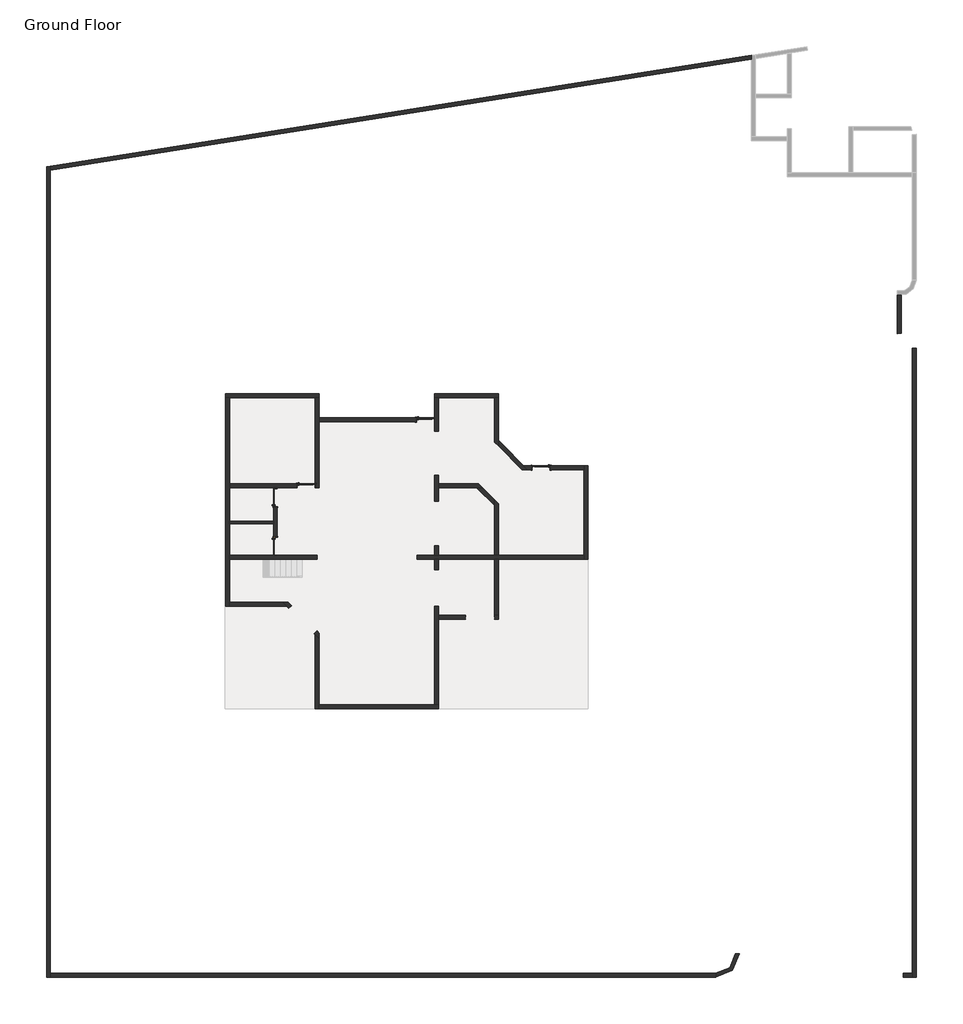
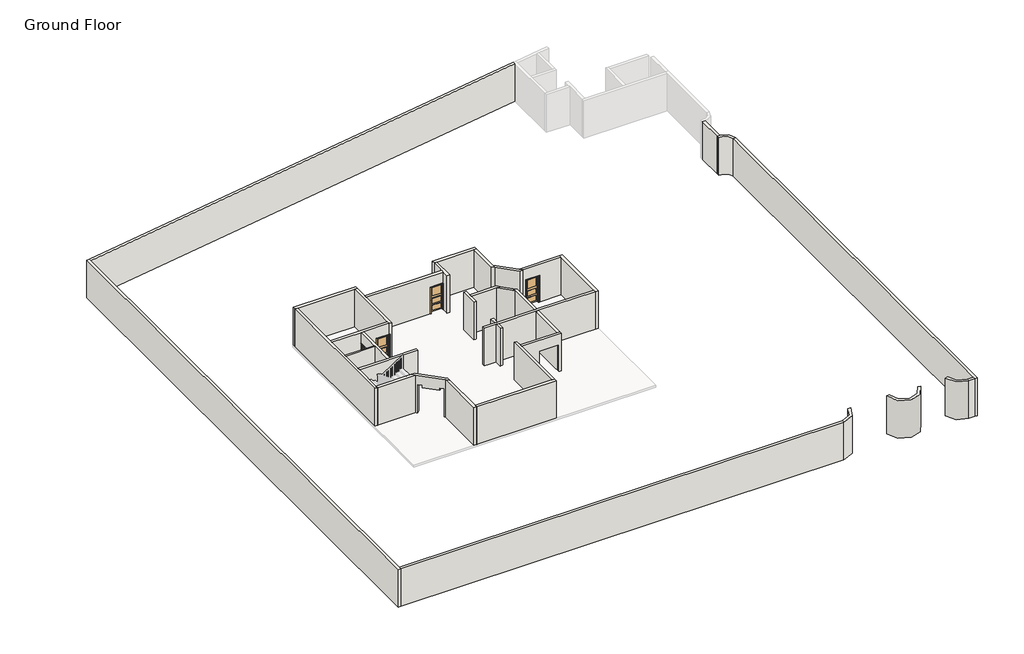
# One storey, part 1 of 2: 37 walls, 5 doors.
"""IFC4 building model written with IfcOpenShell, lengths in millimetres."""

from ifc_helpers import new_model, si_unit, point, frame, frame_2d, origin, origin_with_axes, place, context, project, spatial, polyline, circle_curve, trimmed, segment, composite_curve, outline, extrude, faceted_brep, transform, mapped, element, save
from ifc_brep_helpers import plane_surface, cylinder_surface, revolved_surface, advanced_brep
from components import door_9c4ddfbd, door_1a936fe1, door_721a2355, door_ac5ca1ae

model = new_model("IFC4")

# Units and contexts
model_context = context("Model", 3, world=origin())
ifc_project = project(units=[si_unit("LENGTHUNIT", "METRE", prefix="MILLI")], contexts=[model_context])

# Site, building, storey
site = spatial("IfcSite", under=ifc_project)
building = spatial("IfcBuilding", under=site)
storey = spatial("IfcBuildingStorey", under=building, Name="Ground Floor", Elevation=0.0)

# Doors
placement = place(None, origin())
door_shape = door_9c4ddfbd(model_context)
element("IfcDoor", 1, ObjectType="Door-Interior-Single-1_Panel-Wood : 36\" x 84\"", at=placement, inside=storey, context=model_context, shape_type="MappedRepresentation", body=[
    mapped(door_shape, transform((-23510.5118183, 2144.5392873, 0.0), x_axis=(0.0, 1.0, 0.0), y_axis=(-1.0, 0.0, 0.0), z_axis=(0.0, 0.0, 1.0))),
])
door_2_shape = door_1a936fe1(model_context)
element("IfcDoor", 2, ObjectType="Door-Interior-Single-1_Panel-Wood : 36\" x 84\"", at=placement, inside=storey, context=model_context, shape_type="MappedRepresentation", body=[
    mapped(door_2_shape, transform((-23510.5118183, -342.9715416, 0.0), x_axis=(0.0, -1.0, 0.0), y_axis=(1.0, 0.0, 0.0), z_axis=(0.0, 0.0, 1.0))),
])
door_3_shape = door_721a2355(model_context)
element("IfcDoor", 3, ObjectType="Door-Interior-Single-3_Panel_Vert-Wood : 3' x 6'11\" D1", at=placement, inside=storey, context=model_context, shape_type="MappedRepresentation", body=[
    mapped(door_3_shape, transform((-21930.4431154, 2757.3142873, 0.0), x_axis=(1.0, 0.0, 0.0), y_axis=(0.0, 1.0, 0.0), z_axis=(0.0, 0.0, 1.0))),
])
element("IfcDoor", 4, ObjectType="Door-Interior-Single-3_Panel_Vert-Wood : 3' x 6'11\" D1", at=placement, inside=storey, context=model_context, shape_type="MappedRepresentation", body=[
    mapped(door_3_shape, transform((-15845.1112935, 6113.4026825, 0.0), x_axis=(1.0, 0.0, 0.0), y_axis=(0.0, 1.0, 0.0), z_axis=(0.0, 0.0, 1.0))),
])
door_4_shape = door_ac5ca1ae(model_context)
element("IfcDoor", 5, ObjectType="Door-Interior-Single-3_Panel_Vert-Wood : 3' x 6'11\" D1", at=placement, inside=storey, context=model_context, shape_type="MappedRepresentation", body=[
    mapped(door_4_shape, transform((-9949.3197767, 3672.6109048, 0.0), x_axis=(-1.0, 0.0, 0.0), y_axis=(0.0, -1.0, 0.0), z_axis=(0.0, 0.0, 1.0))),
])

# Walls
element("IfcWall", 6, ObjectType="Generic - 0' - 4 15/16\"", at=placement, inside=storey, context=model_context, shape_type="SweptSolid", body=[
    extrude(outline(polyline([(-23608.9368183, 805.292672), (-25842.0443119, 805.292672), (-25842.0443119, 930.705172), (-23608.9368183, 930.705172), (-23608.9368183, 805.292672)])), origin_with_axes(), (0.0, 0.0, 1.0), 3048.0),
])
element("IfcWall", 7, ObjectType="Generic - 0' - 7 15/16\"", at=placement, inside=storey, context=model_context, shape_type="Brep", body=[
    faceted_brep([(9195.0010201, -22328.4007574, 0.0), (9195.0010201, 9753.6969485, 0.0), (9195.0010201, 9753.6969485, 3048.0), (9195.0010201, -22328.4007574, 3048.0), (8993.3885201, -22328.4007574, 0.0), (8993.3885201, -22328.4007574, 3048.0), (8993.3885201, -22126.7882574, 3048.0), (8993.3885201, 9747.3880188, 3048.0), (8993.3885201, 9747.3880188, 0.0), (8993.3885201, -22126.7882574, 0.0)], [[[0, 1, 2, 3]], [[4, 5, 6, 7, 8, 9]], [[1, 0, 4, 9, 8]], [[3, 2, 7, 6, 5]], [[2, 1, 8, 7]], [[0, 3, 5, 4]]]),
])
element("IfcWall", 8, ObjectType="Generic - 0' - 7 15/16\"", at=placement, inside=storey, context=model_context, shape_type="AdvancedBrep", body=[
    advanced_brep(
    [(9195.0010201, 9753.6969485, 3048.0), (8420.3375232, 10522.820987, 3048.0), (8218.7317611, 10508.1549201, 3048.0), (8218.7317611, 10301.2352695, 3048.0), (8993.3885201, 9747.3880188, 3048.0), (9195.0010201, 9753.6969485, 0.0), (8993.3885201, 9747.3880188, 0.0), (8218.7317611, 10301.2352695, 0.0), (8218.7317611, 10508.1549201, 0.0), (8420.3375232, 10522.820987, 0.0)],
    [
        (0, 1, circle_curve(frame((8378.4275035, 9705.9257341, 3048.0), z_axis=(0.0, 0.0, 1.0), x_axis=(1.0, 0.0, 0.0)), 817.9696798)),
        (1, 2, circle_curve(frame((8378.4275035, 9705.9257341, 3048.0), z_axis=(0.0, 0.0, 1.0), x_axis=(1.0, 0.0, 0.0)), 817.9696229)),
        (2, 3),
        (3, 4, circle_curve(frame((8378.4275035, 9705.9257341, 3048.0), z_axis=(0.0, 0.0, -1.0), x_axis=(1.0, 0.0, 0.0)), 616.3571798)),
        (4, 0),
        (5, 6),
        (6, 7, circle_curve(frame((8378.4275035, 9705.9257341, 0.0), z_axis=(0.0, 0.0, 1.0), x_axis=(1.0, 0.0, 0.0)), 616.3571798)),
        (7, 8),
        (8, 9, circle_curve(frame((8378.4275035, 9705.9257341, 0.0), z_axis=(0.0, 0.0, -1.0), x_axis=(1.0, 0.0, 0.0)), 817.9696798)),
        (9, 5, circle_curve(frame((8378.4275035, 9705.9257341, 0.0), z_axis=(0.0, 0.0, -1.0), x_axis=(1.0, 0.0, 0.0)), 817.9696229)),
        (0, 5),
        (8, 2),
        (3, 7),
        (6, 4),
    ],
    [
        plane_surface(frame((9196.3971832, 9705.9257341, 3048.0), z_axis=(0.0, 0.0, 1.0), x_axis=(0.0, 1.0, 0.0))),
        plane_surface(frame((9196.3971832, 9705.9257341, 0.0), z_axis=(0.0, 0.0, -1.0), x_axis=(0.0, -1.0, 0.0))),
        cylinder_surface(frame((8378.4275035, 9705.9257341, 0.0), z_axis=(0.0, 0.0, 1.0), x_axis=(1.0, 0.0, 0.0)), 817.9696798),
        revolved_surface(polyline([(8994.784683299999, 9705.9257341, 0.0), (8994.784683299999, 9705.9257341, 3048.0)]), (8378.4275035, 9705.9257341, 0.0), (0.0, 0.0, -1.0)),
        plane_surface(frame((8993.3885201, 9747.3880188, 0.0), z_axis=(0.03127704426469031, -0.9995107535699977, 0.0), x_axis=(0.9995107535699977, 0.03127704426469031, 0.0))),
        plane_surface(frame((8218.7317611, 12658.7719349, 0.0), z_axis=(-1.0, 0.0, 0.0), x_axis=(0.0, -1.0, 0.0))),
    ],
    [
        (0, [[1, 2, 3, 4, 5]]),
        (1, [[6, 7, 8, 9, 10]]),
        (2, [[-2, -1, 11, -10, -9, 12]]),
        (3, [[-4, 13, -7, 14]]),
        (4, [[-5, -14, -6, -11]]),
        (5, [[-3, -12, -8, -13]]),
    ],
),
])
element("IfcWall", 9, ObjectType="Generic - 0' - 7 15/16\"", at=placement, inside=storey, context=model_context, shape_type="SweptSolid", body=[
    extrude(outline(composite_curve([segment(polyline([(8218.7317611, 10508.1549201), (8218.7317611, 12472.8269263)]), True, "CONTINUOUS"), segment(trimmed(circle_curve(frame_2d((8381.1692405, 13271.1676702)), 814.6986425), [point((8218.7317611, 12472.8269263))], [point((8420.3442611, 12457.4114439))], True, "CARTESIAN"), True, "CONTINUOUS"), segment(polyline([(8420.3442611, 12457.4114439), (8420.3442611, 10522.8206982)]), True, "CONTINUOUS"), segment(trimmed(circle_curve(frame_2d((8378.4275035, 9705.9257341)), 817.9696798), [point((8420.3442611, 10522.8206982))], [point((8218.7317611, 10508.1549201))], True, "CARTESIAN"), True, "CONTINUOUS")], self_intersect=False)), origin_with_axes(), (0.0, 0.0, 1.0), 3048.0),
])
element("IfcWall", 10, ObjectType="Generic - 0' - 7 15/16\"", at=placement, inside=storey, context=model_context, shape_type="SweptSolid", body=[
    extrude(outline(polyline([(8993.3885201, -22328.4007574), (8533.7347238, -22328.4007574), (8535.4479834, -22126.7882574), (8993.3885201, -22126.7882574), (8993.3885201, -22328.4007574)])), origin_with_axes(), (0.0, 0.0, 1.0), 3048.0),
])
element("IfcWall", 11, ObjectType="Generic - 0' - 7 15/16\"", at=placement, inside=storey, context=model_context, shape_type="SweptSolid", body=[
    extrude(outline(composite_curve([segment(polyline([(7335.4391325, -21276.4548413), (7534.9019602, -21247.0919307)]), True, "CONTINUOUS"), segment(trimmed(circle_curve(frame_2d((8553.7677892, -21097.104755)), 1029.8464596), [point((7534.9019602, -21247.0919307))], [point((8535.4479834, -22126.7882574))], True, "CARTESIAN"), True, "CONTINUOUS"), segment(polyline([(8535.4479834, -22126.7882574), (8533.7347238, -22328.4007574)]), True, "CONTINUOUS"), segment(trimmed(circle_curve(frame_2d((8553.7677892, -21097.104755)), 1231.4589596), [point((8533.7347238, -22328.4007574))], [point((7335.4391325, -21276.4548413))], False, "CARTESIAN"), True, "CONTINUOUS")], self_intersect=False)), origin_with_axes(), (0.0, 0.0, 1.0), 3048.0),
])
element("IfcWall", 12, ObjectType="Generic - 0' - 7 15/16\"", at=placement, inside=storey, context=model_context, shape_type="SweptSolid", body=[
    extrude(outline(composite_curve([segment(polyline([(2932.0157835, -21122.0907213), (3133.3995752, -21112.4902743)]), True, "CONTINUOUS"), segment(trimmed(circle_curve(frame_2d((4193.0797295, -21061.9727873)), 1060.8836156), [point((3133.3995752, -21112.4902743))], [point((5237.6872867, -21247.0919307))], True, "CARTESIAN"), True, "CONTINUOUS"), segment(polyline([(5237.6872867, -21247.0919307), (5436.2066512, -21282.2723527)]), True, "CONTINUOUS"), segment(trimmed(circle_curve(frame_2d((4193.0797295, -21061.9727873)), 1262.4961156), [point((5436.2066512, -21282.2723527))], [point((2932.0157835, -21122.0907213))], False, "CARTESIAN"), True, "CONTINUOUS")], self_intersect=False)), origin_with_axes(), (0.0, 0.0, 1.0), 3048.0),
])
element("IfcWall", 13, ObjectType="Generic - 0' - 7 15/16\"", at=placement, inside=storey, context=model_context, shape_type="SweptSolid", body=[
    extrude(outline(composite_curve([segment(polyline([(-1043.7652203, -22328.1084547), (-1043.7652203, -22126.4959547)]), True, "CONTINUOUS"), segment(trimmed(circle_curve(frame_2d((-1043.7652203, -21112.4902743)), 1014.0056804), [point((-1043.7652203, -22126.4959547))], [point((-29.7595399, -21112.4902743))], True, "CARTESIAN"), True, "CONTINUOUS"), segment(polyline([(-29.7595399, -21112.4902743), (171.8529601, -21112.4902743)]), True, "CONTINUOUS"), segment(trimmed(circle_curve(frame_2d((-1043.7652203, -21112.4902743)), 1215.6181804), [point((171.8529601, -21112.4902743))], [point((-1043.7652203, -22328.1084547))], False, "CARTESIAN"), True, "CONTINUOUS")], self_intersect=False)), origin_with_axes(), (0.0, 0.0, 1.0), 3048.0),
])
element("IfcWall", 14, ObjectType="Generic - 0' - 7 15/16\"", at=placement, inside=storey, context=model_context, shape_type="Brep", body=[
    faceted_brep([(-35183.4613906, 19002.9774571, 0.0), (-35183.4613906, -22328.4007574, 0.0), (-35183.4613906, -22328.4007574, 3048.0), (-35183.4613906, 19002.9774571, 3048.0), (-34981.8488906, 19034.9188254, 0.0), (-34981.8488906, 19034.9188254, 3048.0), (-34981.8488906, 18830.7917788, 3048.0), (-34981.8488906, -22328.4007574, 3048.0), (-34981.8488906, -22328.4007574, 0.0), (-34981.8488906, 18830.7917788, 0.0)], [[[0, 1, 2, 3]], [[4, 5, 6, 7, 8, 9]], [[1, 0, 4, 9, 8]], [[2, 1, 8, 7]], [[3, 2, 7, 6, 5]], [[0, 3, 5, 4]]]),
])
element("IfcWall", 15, ObjectType="Generic - 0' - 7 15/16\"", at=placement, inside=storey, context=model_context, shape_type="SweptSolid", body=[
    extrude(outline(polyline([(-1034.7920906, -22328.4007574), (-34981.5566627, -22328.4007574), (-34981.5566627, -22126.7882574), (-1034.7920906, -22126.7882574), (-1034.7920906, -22328.4007574)])), origin_with_axes(), (0.0, 0.0, 1.0), 3048.0),
])
element("IfcWall", 16, ObjectType="Generic - 0' - 7 15/16\"", at=placement, inside=storey, context=model_context, shape_type="Brep", body=[
    faceted_brep([(787.1202427, 24701.7788574, 0.0), (-34981.8488906, 19034.9188254, 0.0), (-34981.8488906, 19034.9188254, 3048.0), (787.1202427, 24701.7788574, 3048.0), (787.1202427, 24497.6518108, 0.0), (787.1202427, 24497.6518108, 3048.0), (-34981.8488906, 18830.7917788, 3048.0), (-34981.8488906, 18830.7917788, 0.0), (787.1202427, 24699.1003289, 0.0), (787.1202427, 24699.1003289, 3048.0)], [[[0, 1, 2, 3]], [[4, 5, 6, 7]], [[1, 0, 8, 4, 7]], [[3, 2, 6, 5, 9]], [[0, 3, 9, 5, 4, 8]], [[2, 1, 7, 6]]]),
])
element("IfcWall", 17, ObjectType="Generic - 0' - 7 15/16\"", at=placement, inside=storey, context=model_context, shape_type="Brep", body=[
    faceted_brep([(-25842.0443119, -800.9652916, 3048.0), (-23608.9368183, -800.9652916, 3048.0), (-23405.7368183, -800.9652916, 3048.0), (-21373.2387805, -800.9652916, 3048.0), (-21373.2387805, -800.9652916, 0.0), (-23405.7368183, -800.9652916, 0.0), (-23405.7368183, -800.9652916, 2159.0), (-23608.9368183, -800.9652916, 2159.0), (-23608.9368183, -800.9652916, 0.0), (-25842.0443119, -800.9652916, 0.0), (-25842.0443119, -1002.5777916, 0.0), (-21373.2387805, -1002.5777916, 0.0), (-21373.2387805, -1002.5777916, 3048.0), (-25842.0443119, -1002.5777916, 3048.0), (-23608.9368183, -825.5715416, 0.0), (-23405.7368183, -825.5715416, 0.0), (-23608.9368183, -825.5715416, 2159.0), (-23405.7368183, -825.5715416, 2159.0)], [[[0, 1, 2, 3, 4, 5, 6, 7, 8, 9]], [[10, 11, 12, 13]], [[11, 10, 9, 8, 14, 15, 5, 4]], [[3, 2, 1, 0, 13, 12]], [[4, 3, 12, 11]], [[0, 9, 10, 13]], [[16, 14, 8, 7]], [[15, 17, 6, 5]], [[14, 16, 17, 15]], [[17, 16, 7, 6]]]),
])
element("IfcWall", 18, ObjectType="Generic - 8\"", at=placement, inside=storey, context=model_context, shape_type="Brep", body=[
    faceted_brep([(-21270.0431154, 7427.7381656, 0.0), (-26045.2443119, 7427.7381656, 0.0), (-26045.2443119, 7427.7381656, 3048.0), (-21270.0431154, 7427.7381656, 3048.0), (-21270.0431154, 7224.5381656, 0.0), (-21270.0431154, 7224.5381656, 3048.0), (-21473.2431154, 7224.5381656, 3048.0), (-25842.0443119, 7224.5381656, 3048.0), (-26045.2443119, 7224.5381656, 3048.0), (-26045.2443119, 7224.5381656, 0.0), (-25842.0443119, 7224.5381656, 0.0), (-21473.2431154, 7224.5381656, 0.0)], [[[0, 1, 2, 3]], [[4, 5, 6, 7, 8, 9, 10, 11]], [[1, 0, 4, 11, 10, 9]], [[3, 2, 8, 7, 6, 5]], [[2, 1, 9, 8]], [[0, 3, 5, 4]]]),
])
element("IfcWall", 19, ObjectType="Generic - 8\"", at=placement, inside=storey, context=model_context, shape_type="Brep", body=[
    faceted_brep([(-25842.0443119, -3391.115973, 0.0), (-25842.0443119, -3187.915973, 0.0), (-25842.0443119, -1002.5777916, 0.0), (-25842.0443119, -800.9652916, 0.0), (-25842.0443119, 805.292672, 0.0), (-25842.0443119, 930.705172, 0.0), (-25842.0443119, 2652.5392873, 0.0), (-25842.0443119, 2855.7392873, 0.0), (-25842.0443119, 7224.5381656, 0.0), (-25842.0443119, 7224.5381656, 3048.0), (-25842.0443119, 2855.7392873, 3048.0), (-25842.0443119, 2652.5392873, 3048.0), (-25842.0443119, 930.705172, 3048.0), (-25842.0443119, 805.292672, 3048.0), (-25842.0443119, -800.9652916, 3048.0), (-25842.0443119, -1002.5777916, 3048.0), (-25842.0443119, -3187.915973, 3048.0), (-25842.0443119, -3391.115973, 3048.0), (-26045.2443119, -3391.115973, 0.0), (-26045.2443119, -3391.115973, 3048.0), (-26045.2443119, 7224.5381656, 3048.0), (-26045.2443119, 7224.5381656, 0.0)], [[[0, 1, 2, 3, 4, 5, 6, 7, 8, 9, 10, 11, 12, 13, 14, 15, 16, 17]], [[18, 19, 20, 21]], [[8, 7, 6, 5, 4, 3, 2, 1, 0, 18, 21]], [[17, 16, 15, 14, 13, 12, 11, 10, 9, 20, 19]], [[9, 8, 21, 20]], [[0, 17, 19, 18]]]),
])
element("IfcWall", 20, ObjectType="Generic - 8\"", at=placement, inside=storey, context=model_context, shape_type="Brep", body=[
    faceted_brep([(-25842.0443119, 2855.7392873, 3048.0), (-21473.2431154, 2855.7392873, 3048.0), (-21473.2431154, 2855.7392873, 2133.6), (-22413.0431154, 2855.7392873, 2133.6), (-22413.0431154, 2855.7392873, 0.0), (-25842.0443119, 2855.7392873, 0.0), (-21473.2431154, 2652.5392873, 3048.0), (-23405.7368183, 2652.5392873, 3048.0), (-23608.9368183, 2652.5392873, 3048.0), (-25842.0443119, 2652.5392873, 3048.0), (-25842.0443119, 2652.5392873, 0.0), (-23608.9368183, 2652.5392873, 0.0), (-23405.7368183, 2652.5392873, 0.0), (-22413.0431154, 2652.5392873, 0.0), (-22413.0431154, 2652.5392873, 2133.6), (-21473.2431154, 2652.5392873, 2133.6)], [[[0, 1, 2, 3, 4, 5]], [[6, 7, 8, 9, 10, 11, 12, 13, 14, 15]], [[10, 5, 4, 13, 12, 11]], [[1, 0, 9, 8, 7, 6]], [[0, 5, 10, 9]], [[1, 6, 15, 2]], [[14, 3, 2, 15]], [[3, 14, 13, 4]]]),
])
element("IfcWall", 21, ObjectType="Generic - 8\"", at=placement, inside=storey, context=model_context, shape_type="Brep", body=[
    faceted_brep([(-21270.0431154, 2652.5392873, 0.0), (-21270.0431154, 6008.6276825, 0.0), (-21270.0431154, 6211.8276825, 0.0), (-21270.0431154, 7224.5381656, 0.0), (-21270.0431154, 7224.5381656, 3048.0), (-21270.0431154, 6211.8276825, 3048.0), (-21270.0431154, 6008.6276825, 3048.0), (-21270.0431154, 2652.5392873, 3048.0), (-21473.2431154, 2652.5392873, 3048.0), (-21473.2431154, 2855.7392873, 3048.0), (-21473.2431154, 7224.5381656, 3048.0), (-21473.2431154, 7224.5381656, 0.0), (-21473.2431154, 2855.7392873, 0.0), (-21473.2431154, 2855.7392873, 2133.6), (-21473.2431154, 2652.5392873, 2133.6), (-21447.8431154, 2652.5392873, 0.0), (-21447.8431154, 2855.7392873, 0.0), (-21447.8431154, 2652.5392873, 2133.6), (-21447.8431154, 2855.7392873, 2133.6)], [[[0, 1, 2, 3, 4, 5, 6, 7]], [[8, 9, 10, 11, 12, 13, 14]], [[3, 2, 1, 0, 15, 16, 12, 11]], [[7, 6, 5, 4, 10, 9, 8]], [[4, 3, 11, 10]], [[0, 7, 8, 14, 17, 15]], [[16, 18, 13, 12]], [[18, 16, 15, 17]], [[18, 17, 14, 13]]]),
])
element("IfcWall", 22, ObjectType="Generic - 8\"", at=placement, inside=storey, context=model_context, shape_type="SweptSolid", body=[
    extrude(outline(polyline([(3048.0, -15387.9112935), (3048.0, -21270.0431154), (0.0, -21270.0431154), (0.0, -16327.7112935), (2133.6, -16327.7112935), (2133.6, -15387.9112935), (3048.0, -15387.9112935)])), frame((0.0, 6008.6276825, 0.0), z_axis=(0.0, 1.0, 0.0), x_axis=(0.0, 0.0, 1.0)), (0.0, 0.0, 1.0), 203.2),
])
element("IfcWall", 23, ObjectType="Generic - 8\"", at=placement, inside=storey, context=model_context, shape_type="SweptSolid", body=[
    extrude(outline(polyline([(-15177.0356792, 7224.5381656), (-15177.0356792, 5525.355182), (-15380.2356792, 5525.355182), (-15380.2356792, 7224.5381656), (-15177.0356792, 7224.5381656)])), origin_with_axes(), (0.0, 0.0, 1.0), 3048.0),
])
element("IfcWall", 24, ObjectType="Generic - 8\"", at=placement, inside=storey, context=model_context, shape_type="Brep", body=[
    faceted_brep([(-12130.529643, 7427.7381656, 0.0), (-15383.4246912, 7427.7381656, 0.0), (-15383.4246912, 7427.7381656, 3048.0), (-12130.529643, 7427.7381656, 3048.0), (-12130.529643, 7224.5381656, 0.0), (-12130.529643, 7224.5381656, 3048.0), (-12133.7209731, 7224.5381656, 3048.0), (-12336.9209731, 7224.5381656, 3048.0), (-15177.0356792, 7224.5381656, 3048.0), (-15380.2356792, 7224.5381656, 3048.0), (-15383.4246912, 7224.5381656, 3048.0), (-15383.4246912, 7224.5381656, 0.0), (-15380.2356792, 7224.5381656, 0.0), (-15177.0356792, 7224.5381656, 0.0), (-12336.9209731, 7224.5381656, 0.0), (-12133.7209731, 7224.5381656, 0.0)], [[[0, 1, 2, 3]], [[4, 5, 6, 7, 8, 9, 10, 11, 12, 13, 14, 15]], [[1, 0, 4, 15, 14, 13, 12, 11]], [[2, 1, 11, 10]], [[3, 2, 10, 9, 8, 7, 6, 5]], [[0, 3, 5, 4]]]),
])
element("IfcWall", 25, ObjectType="Generic - 8\"", at=placement, inside=storey, context=model_context, shape_type="Brep", body=[
    faceted_brep([(-12133.7209731, 4774.4410298, 0.0), (-10927.1158481, 3567.8359048, 0.0), (-10927.1158481, 3567.8359048, 3048.0), (-12133.7209731, 4774.4410298, 3048.0), (-12133.7209731, 5061.8092257, 0.0), (-12133.7209731, 5061.8092257, 3048.0), (-10842.9476523, 3771.0359048, 3048.0), (-10639.7476523, 3567.8359048, 3048.0), (-10639.7476523, 3567.8359048, 0.0), (-10842.9476523, 3771.0359048, 0.0)], [[[0, 1, 2, 3]], [[4, 5, 6, 7, 8, 9]], [[1, 0, 4, 9, 8]], [[3, 2, 7, 6, 5]], [[2, 1, 8, 7]], [[0, 3, 5, 4]]]),
])
element("IfcWall", 26, ObjectType="Generic - 8\"", at=placement, inside=storey, context=model_context, shape_type="Brep", body=[
    faceted_brep([(-12336.9209731, 7224.5381656, 0.0), (-12336.9209731, 4977.6410298, 0.0), (-12336.9209731, 4977.6410298, 3048.0), (-12336.9209731, 7224.5381656, 3048.0), (-12133.7209731, 7224.5381656, 0.0), (-12133.7209731, 7224.5381656, 3048.0), (-12133.7209731, 5061.8092257, 3048.0), (-12133.7209731, 4774.4410298, 3048.0), (-12133.7209731, 4774.4410298, 0.0), (-12133.7209731, 5061.8092257, 0.0)], [[[0, 1, 2, 3]], [[4, 5, 6, 7, 8, 9]], [[1, 0, 4, 9, 8]], [[3, 2, 7, 6, 5]], [[2, 1, 8, 7]], [[0, 3, 5, 4]]]),
])
element("IfcWall", 27, ObjectType="Generic - 8\"", at=placement, inside=storey, context=model_context, shape_type="Brep", body=[
    faceted_brep([(-7764.9197767, 3771.0359048, 0.0), (-7764.9197767, 3567.8359048, 0.0), (-7764.9197767, -800.9652916, 0.0), (-7764.9197767, -1004.1652916, 0.0), (-7764.9197767, -1004.1652916, 3048.0), (-7764.9197767, -800.9652916, 3048.0), (-7764.9197767, 3567.8359048, 3048.0), (-7764.9197767, 3771.0359048, 3048.0), (-7561.7197767, 3771.0359048, 0.0), (-7561.7197767, 3771.0359048, 3048.0), (-7561.7197767, -1004.1652916, 3048.0), (-7561.7197767, -1004.1652916, 0.0)], [[[0, 1, 2, 3, 4, 5, 6, 7]], [[8, 9, 10, 11]], [[3, 2, 1, 0, 8, 11]], [[7, 6, 5, 4, 10, 9]], [[4, 3, 11, 10]], [[0, 7, 9, 8]]]),
])
element("IfcWall", 28, ObjectType="Generic - 8\"", at=placement, inside=storey, context=model_context, shape_type="Brep", body=[
    faceted_brep([(-7764.9197767, -800.9652916, 0.0), (-12130.529643, -800.9652916, 0.0), (-12333.729643, -800.9652916, 0.0), (-15177.0356792, -800.9652916, 0.0), (-15380.2356792, -800.9652916, 0.0), (-16280.7750494, -800.9652916, 0.0), (-16280.7750494, -800.9652916, 3048.0), (-15380.2356792, -800.9652916, 3048.0), (-15177.0356792, -800.9652916, 3048.0), (-12333.729643, -800.9652916, 3048.0), (-12130.529643, -800.9652916, 3048.0), (-7764.9197767, -800.9652916, 3048.0), (-7764.9197767, -1004.1652916, 0.0), (-7764.9197767, -1004.1652916, 3048.0), (-12130.529643, -1004.1652916, 3048.0), (-12333.729643, -1004.1652916, 3048.0), (-15177.0356792, -1004.1652916, 3048.0), (-15380.2356792, -1004.1652916, 3048.0), (-16280.7750494, -1004.1652916, 3048.0), (-16280.7750494, -1004.1652916, 0.0), (-15380.2356792, -1004.1652916, 0.0), (-15177.0356792, -1004.1652916, 0.0), (-12333.729643, -1004.1652916, 0.0), (-12130.529643, -1004.1652916, 0.0)], [[[0, 1, 2, 3, 4, 5, 6, 7, 8, 9, 10, 11]], [[12, 13, 14, 15, 16, 17, 18, 19, 20, 21, 22, 23]], [[5, 4, 3, 2, 1, 0, 12, 23, 22, 21, 20, 19]], [[6, 5, 19, 18]], [[11, 10, 9, 8, 7, 6, 18, 17, 16, 15, 14, 13]], [[0, 11, 13, 12]]]),
])
element("IfcWall", 29, ObjectType="Generic - 8\"", at=placement, inside=storey, context=model_context, shape_type="Brep", body=[
    faceted_brep([(-12130.529643, -800.9652916, 0.0), (-12130.529643, 1838.499171, 0.0), (-12130.529643, 1838.499171, 3048.0), (-12130.529643, -800.9652916, 3048.0), (-12333.729643, -800.9652916, 0.0), (-12333.729643, -800.9652916, 3048.0), (-12333.729643, 1754.3309751, 3048.0), (-12333.729643, 2041.699171, 3048.0), (-12333.729643, 2041.699171, 0.0), (-12333.729643, 1754.3309751, 0.0)], [[[0, 1, 2, 3]], [[4, 5, 6, 7, 8, 9]], [[1, 0, 4, 9, 8]], [[3, 2, 7, 6, 5]], [[0, 3, 5, 4]], [[2, 1, 8, 7]]]),
])
element("IfcWall", 30, ObjectType="Generic - 8\"", at=placement, inside=storey, context=model_context, shape_type="SweptSolid", body=[
    extrude(outline(polyline([(-12130.529643, -1004.1652916), (-12130.529643, -3846.1737377), (-12333.729643, -3846.1737377), (-12333.729643, -1004.1652916), (-12130.529643, -1004.1652916)])), origin_with_axes(), (0.0, 0.0, 1.0), 3048.0),
])
element("IfcWall", 31, ObjectType="Generic - 8\"", at=placement, inside=storey, context=model_context, shape_type="Brep", body=[
    faceted_brep([(-12130.529643, -4049.3737377, 3048.0), (-15180.2246912, -4049.3737377, 3048.0), (-15180.2246912, -4049.3737377, 0.0), (-13812.829643, -4049.3737377, 0.0), (-13812.829643, -4049.3737377, 2189.5), (-12327.829643, -4049.3737377, 2189.5), (-12327.829643, -4049.3737377, 0.0), (-12130.529643, -4049.3737377, 0.0), (-15180.2246912, -3846.1737377, 3048.0), (-12333.729643, -3846.1737377, 3048.0), (-12130.529643, -3846.1737377, 3048.0), (-12130.529643, -3846.1737377, 0.0), (-12327.829643, -3846.1737377, 0.0), (-12327.829643, -3846.1737377, 2189.5), (-13812.829643, -3846.1737377, 2189.5), (-13812.829643, -3846.1737377, 0.0), (-15180.2246912, -3846.1737377, 0.0), (-13812.829643, -3952.3737377, 0.0), (-13827.829643, -3952.3737377, 0.0), (-13827.829643, -4029.3737377, 0.0), (-13812.829643, -4029.3737377, 0.0), (-12327.829643, -4029.3737377, 0.0), (-12312.829643, -4029.3737377, 0.0), (-12312.829643, -3952.3737377, 0.0), (-12327.829643, -3952.3737377, 0.0), (-13812.829643, -4029.3737377, 2189.5), (-12327.829643, -4029.3737377, 2189.5), (-13827.829643, -4029.3737377, 2204.5), (-12312.829643, -4029.3737377, 2204.5), (-13827.829643, -3952.3737377, 2204.5), (-13812.829643, -3952.3737377, 2189.5), (-12327.829643, -3952.3737377, 2189.5), (-12312.829643, -3952.3737377, 2204.5)], [[[0, 1, 2, 3, 4, 5, 6, 7]], [[8, 9, 10, 11, 12, 13, 14, 15, 16]], [[2, 16, 15, 17, 18, 19, 20, 3]], [[11, 7, 6, 21, 22, 23, 24, 12]], [[1, 0, 10, 9, 8]], [[2, 1, 8, 16]], [[0, 7, 11, 10]], [[20, 25, 4, 3]], [[26, 21, 6, 5]], [[25, 26, 5, 4]], [[25, 20, 19, 27, 28, 22, 21, 26]], [[27, 19, 18, 29]], [[29, 18, 17, 30, 31, 24, 23, 32]], [[28, 27, 29, 32]], [[22, 28, 32, 23]], [[30, 17, 15, 14]], [[24, 31, 13, 12]], [[31, 30, 14, 13]]]),
])
element("IfcWall", 32, ObjectType="Generic - 8\"", at=placement, inside=storey, context=model_context, shape_type="Brep", body=[
    faceted_brep([(-15383.4246912, -3394.3072284, 0.0), (-15383.4246912, -8414.9836039, 0.0), (-15383.4246912, -8414.9836039, 3048.0), (-15383.4246912, -3394.3072284, 3048.0), (-15180.2246912, -3394.3072284, 0.0), (-15180.2246912, -3394.3072284, 3048.0), (-15180.2246912, -3846.1737377, 3048.0), (-15180.2246912, -4049.3737377, 3048.0), (-15180.2246912, -8414.9836039, 3048.0), (-15180.2246912, -8414.9836039, 0.0), (-15180.2246912, -4049.3737377, 0.0), (-15180.2246912, -3846.1737377, 0.0)], [[[0, 1, 2, 3]], [[4, 5, 6, 7, 8, 9, 10, 11]], [[1, 0, 4, 11, 10, 9]], [[3, 2, 8, 7, 6, 5]], [[0, 3, 5, 4]], [[2, 1, 9, 8]]]),
])
element("IfcWall", 33, ObjectType="Generic - 8\"", at=placement, inside=storey, context=model_context, shape_type="Brep", body=[
    faceted_brep([(-15180.2246912, -8414.9836039, 0.0), (-15383.4246912, -8414.9836039, 0.0), (-21270.0431154, -8414.9836039, 0.0), (-21270.0431154, -8414.9836039, 3048.0), (-15383.4246912, -8414.9836039, 3048.0), (-15180.2246912, -8414.9836039, 3048.0), (-15180.2246912, -8618.1836039, 0.0), (-15180.2246912, -8618.1836039, 3048.0), (-21270.0431154, -8618.1836039, 3048.0), (-21270.0431154, -8618.1836039, 0.0)], [[[0, 1, 2, 3, 4, 5]], [[6, 7, 8, 9]], [[2, 1, 0, 6, 9]], [[5, 4, 3, 8, 7]], [[3, 2, 9, 8]], [[0, 5, 7, 6]]]),
])
element("IfcWall", 34, ObjectType="Generic - 8\"", at=placement, inside=storey, context=model_context, shape_type="Brep", body=[
    faceted_brep([(-21270.0431154, -8618.1836039, 0.0), (-21270.0431154, -8414.9836039, 0.0), (-21270.0431154, -5059.1070276, 0.0), (-21270.0431154, -5059.1070276, 3048.0), (-21270.0431154, -8414.9836039, 3048.0), (-21270.0431154, -8618.1836039, 3048.0), (-21473.2431154, -8618.1836039, 0.0), (-21473.2431154, -8618.1836039, 3048.0), (-21473.2431154, -4855.9070276, 3048.0), (-21473.2431154, -4855.9070276, 0.0)], [[[0, 1, 2, 3, 4, 5]], [[6, 7, 8, 9]], [[2, 1, 0, 6, 9]], [[5, 4, 3, 8, 7]], [[3, 2, 9, 8]], [[0, 5, 7, 6]]]),
])
element("IfcWall", 35, ObjectType="Generic - 8\"", at=placement, inside=storey, context=model_context, shape_type="SweptSolid", body=[
    extrude(outline(polyline([(-25842.0443119, -3187.915973), (-23141.23417, -3187.915973), (-22938.03417, -3391.115973), (-25842.0443119, -3391.115973), (-25842.0443119, -3187.915973)])), origin_with_axes(), (0.0, 0.0, 1.0), 3048.0),
])
element("IfcWall", 36, ObjectType="Generic - 8\"", at=placement, inside=storey, context=model_context, shape_type="Brep", body=[
    faceted_brep([(-22853.8659741, -3187.915973, 3048.0), (-21270.0431154, -4771.7388317, 3048.0), (-21270.0431154, -4771.7388317, 0.0), (-21385.3381768, -4656.4437704, 0.0), (-21385.3381768, -4656.4437704, 2286.0), (-21600.8643237, -4440.9176235, 2286.0), (-21600.8643237, -4440.9176235, 2108.2), (-22462.9689113, -3578.8130358, 2108.2), (-22462.9689113, -3578.8130358, 2286.0), (-22678.4950582, -3363.2868889, 2286.0), (-22678.4950582, -3363.2868889, 0.0), (-22853.8659741, -3187.915973, 0.0), (-21270.0431154, -5059.1070276, 3048.0), (-21473.2431154, -4855.9070276, 3048.0), (-22938.03417, -3391.115973, 3048.0), (-23141.23417, -3187.915973, 3048.0), (-23141.23417, -3187.915973, 0.0), (-22938.03417, -3391.115973, 0.0), (-22822.1791562, -3506.9709869, 0.0), (-22822.1791562, -3506.9709869, 2286.0), (-22606.6530093, -3722.4971338, 2286.0), (-22606.6530093, -3722.4971338, 2108.2), (-21744.5484216, -4584.6017214, 2108.2), (-21744.5484216, -4584.6017214, 2286.0), (-21529.0222747, -4800.1278683, 2286.0), (-21529.0222747, -4800.1278683, 0.0), (-21473.2431154, -4855.9070276, 0.0), (-21270.0431154, -5059.1070276, 0.0)], [[[0, 1, 2, 3, 4, 5, 6, 7, 8, 9, 10, 11]], [[12, 13, 14, 15, 16, 17, 18, 19, 20, 21, 22, 23, 24, 25, 26, 27]], [[16, 11, 10, 18, 17]], [[2, 27, 26, 25, 3]], [[1, 0, 15, 14, 13, 12]], [[0, 11, 16, 15]], [[2, 1, 12, 27]], [[6, 22, 21, 7]], [[5, 23, 22, 6]], [[24, 4, 3, 25]], [[23, 5, 4, 24]], [[9, 19, 18, 10]], [[20, 8, 7, 21]], [[19, 9, 8, 20]]]),
])
element("IfcWall", 37, ObjectType="Generic - 8\"", at=placement, inside=storey, context=model_context, shape_type="SweptSolid", body=[
    extrude(outline(polyline([(-15380.2356792, -316.3952757), (-15177.0356792, -316.3952757), (-15177.0356792, -800.9652916), (-15380.2356792, -800.9652916), (-15380.2356792, -316.3952757)])), origin_with_axes(), (0.0, 0.0, 1.0), 3048.0),
    extrude(outline(polyline([(-15177.0356792, -1536.7922862), (-15380.2356792, -1536.7922862), (-15380.2356792, -1004.1652916), (-15177.0356792, -1004.1652916), (-15177.0356792, -1536.7922862)])), origin_with_axes(), (0.0, 0.0, 1.0), 3048.0),
])
element("IfcWall", 38, ObjectType="Generic - 8\"", at=placement, inside=storey, context=model_context, shape_type="SweptSolid", body=[
    extrude(outline(polyline([(-15383.4246912, 1953.9000835), (-15383.4246912, 3286.4658888), (-15180.2246912, 3286.4658888), (-15180.2246912, 1953.9000835), (-15383.4246912, 1953.9000835)])), origin_with_axes(), (0.0, 0.0, 1.0), 3048.0),
])
element("IfcWall", 39, ObjectType="Generic - 8\"", at=placement, inside=storey, context=model_context, shape_type="Brep", body=[
    faceted_brep([(-13147.7697593, 2855.7392873, 0.0), (-15177.0356792, 2855.7392873, 0.0), (-15177.0356792, 2855.7392873, 3048.0), (-13147.7697593, 2855.7392873, 3048.0), (-12944.5697593, 2652.5392873, 0.0), (-12944.5697593, 2652.5392873, 3048.0), (-13231.9379551, 2652.5392873, 3048.0), (-15177.0356792, 2652.5392873, 3048.0), (-15177.0356792, 2652.5392873, 0.0), (-13231.9379551, 2652.5392873, 0.0)], [[[0, 1, 2, 3]], [[4, 5, 6, 7, 8, 9]], [[1, 0, 4, 9, 8]], [[2, 1, 8, 7]], [[3, 2, 7, 6, 5]], [[0, 3, 5, 4]]]),
])
element("IfcWall", 40, ObjectType="Generic - 8\"", at=placement, inside=storey, context=model_context, shape_type="SweptSolid", body=[
    extrude(outline(polyline([(-12944.5697593, 2652.5392873), (-12333.729643, 2041.699171), (-12333.729643, 1754.3309751), (-13231.9379551, 2652.5392873), (-12944.5697593, 2652.5392873)])), origin_with_axes(), (0.0, 0.0, 1.0), 3048.0),
])
element("IfcWall", 41, ObjectType="Generic - 8\"", at=placement, inside=storey, context=model_context, shape_type="Brep", body=[
    faceted_brep([(-10842.9476523, 3771.0359048, 3048.0), (-7764.9197767, 3771.0359048, 3048.0), (-7764.9197767, 3771.0359048, 0.0), (-9466.7197767, 3771.0359048, 0.0), (-9466.7197767, 3771.0359048, 2133.6), (-10431.9197767, 3771.0359048, 2133.6), (-10431.9197767, 3771.0359048, 0.0), (-10842.9476523, 3771.0359048, 0.0), (-7764.9197767, 3567.8359048, 3048.0), (-10639.7476523, 3567.8359048, 3048.0), (-10639.7476523, 3567.8359048, 0.0), (-10431.9197767, 3567.8359048, 0.0), (-10431.9197767, 3567.8359048, 2133.6), (-9466.7197767, 3567.8359048, 2133.6), (-9466.7197767, 3567.8359048, 0.0), (-7764.9197767, 3567.8359048, 0.0)], [[[0, 1, 2, 3, 4, 5, 6, 7]], [[8, 9, 10, 11, 12, 13, 14, 15]], [[2, 15, 14, 3]], [[10, 7, 6, 11]], [[1, 0, 9, 8]], [[2, 1, 8, 15]], [[0, 7, 10, 9]], [[5, 12, 11, 6]], [[12, 5, 4, 13]], [[13, 4, 3, 14]]]),
])
element("IfcWall", 42, ObjectType="Generic - 8\"", at=placement, inside=storey, context=model_context, shape_type="Brep", body=[
    faceted_brep([(-23405.7368183, 2652.5392873, 3048.0), (-23405.7368183, -800.9652916, 3048.0), (-23405.7368183, -800.9652916, 2159.0), (-23405.7368183, 139.6284584, 2159.0), (-23405.7368183, 139.6284584, 0.0), (-23405.7368183, 1661.9392873, 0.0), (-23405.7368183, 1661.9392873, 2159.0), (-23405.7368183, 2627.1392873, 2159.0), (-23405.7368183, 2627.1392873, 0.0), (-23405.7368183, 2652.5392873, 0.0), (-23608.9368183, -800.9652916, 3048.0), (-23608.9368183, 805.292672, 3048.0), (-23608.9368183, 930.705172, 3048.0), (-23608.9368183, 2652.5392873, 3048.0), (-23608.9368183, 2652.5392873, 0.0), (-23608.9368183, 2627.1392873, 0.0), (-23608.9368183, 2627.1392873, 2159.0), (-23608.9368183, 1661.9392873, 2159.0), (-23608.9368183, 1661.9392873, 0.0), (-23608.9368183, 930.705172, 0.0), (-23608.9368183, 805.292672, 0.0), (-23608.9368183, 139.6284584, 0.0), (-23608.9368183, 139.6284584, 2159.0), (-23608.9368183, -800.9652916, 2159.0)], [[[0, 1, 2, 3, 4, 5, 6, 7, 8, 9]], [[10, 11, 12, 13, 14, 15, 16, 17, 18, 19, 20, 21, 22, 23]], [[14, 9, 8, 15]], [[18, 5, 4, 21, 20, 19]], [[1, 0, 13, 12, 11, 10]], [[1, 10, 23, 2]], [[0, 9, 14, 13]], [[7, 16, 15, 8]], [[16, 7, 6, 17]], [[17, 6, 5, 18]], [[22, 3, 2, 23]], [[3, 22, 21, 4]]]),
])

save(model, "model.ifc")

# Revit data of these elements
# Type "Door-Interior-Single-1_Panel-Wood : 36\" x 84\""
#   Type Mark = "10"
#   Analytic Construction = "Wooden"
#   Top Rail = 0' - 4 11/16"
#   Thickness = 0' - 1 3/8"
#   Thermal Resistance (R) = 2.5876 (h·ft²·°F)/BTU
#   Swing Angle [instance default] = 90.00°
#   Stiles = 0' - 4 3/4"
#   Rough Width = 3' - 2"
#   Rough Height = 7' - 1"
#   Height = 7' - 0"
#   Width = 3' - 0"
#   Heat Transfer Coefficient (U) = 0.3865 BTU/(h·ft²·°F)
#   Bottom Rail = 0' - 9 1/8"
#   Trim Material = Cherry
#   Panel Material = Cherry
#   Frame Material = Cherry
#   Door Handle Material = Aluminum
#   Visual Light Transmittance = 0
#   Solar Heat Gain Coefficient = 0
#   Wall Closure = (empty or 0)
#   Function = (empty or 0)
# Type "Door-Interior-Single-3_Panel_Vert-Wood : 3' x 6'11\" D1"
#   Type Mark = "9"
#   Analytic Construction = "Wooden"
#   Top Rail = 0' - 4 11/16"
#   Thickness = 0' - 1 3/8"
#   Thermal Resistance (R) = 2.5876 (h·ft²·°F)/BTU
#   Swing Angle [instance default] = 90.00°
#   Stiles = 0' - 4 3/4"
#   Rough Width = 3' - 2"
#   Rough Height = 7' - 0"
#   Intermediate Rail = 0' - 4 1/2"
#   Height = 6' - 11"
#   Width = 3' - 0"
#   Heat Transfer Coefficient (U) = 0.3865 BTU/(h·ft²·°F)
#   Bottom Rail = 0' - 9 1/8"
#   Define Thermal Properties by = 1
#   Trim Material = Cherry
#   Panel Material = Cherry
#   Frame Material = Cherry
#   Door Handle Material = Aluminum
#   Visual Light Transmittance = 0
#   Solar Heat Gain Coefficient = 0
#   Wall Closure = (empty or 0)
#   Function = (empty or 0)
# Type "Generic - 0' - 4 15/16\""
#   Layers, outside or top first: 0' - 4 15/16" no material (function 1)
# Type "Generic - 0' - 7 15/16\""
#   Layers, outside or top first: 0' - 7 15/16" no material (function 1)
# Type "Generic - 8\""
#   Layers, outside or top first: 0' - 8" no material (function 1)
# Elements 1, 2 (IfcDoor, "Door-Interior-Single-1_Panel-Wood : 36\" x 84\"")
#   Swing Angle = 90.00°
#   Phase Created = New Construction
#   Materials on its faces: "Cherry", "Aluminum"
# Elements 3, 4, 5 (IfcDoor, "Door-Interior-Single-3_Panel_Vert-Wood : 3' x 6'11\" D1")
#   Swing Angle = 90.00°
#   Phase Created = New Construction
#   Materials on its faces: "Cherry", "Aluminum"
# Element 6 (IfcWall, "Generic - 0' - 4 15/16\"")
#   Top Offset = 0' - 0"
#   Base Offset = 0' - 0"
#   wall height = 10' - 0"
#   Phase Created = New Construction
#   Base Constraint = Ground Floor
#   Top Constraint = First Floor
#   Materials on its faces: "Default Wall"
# Elements 7, 9, 10, 14, 15, 16, 17 (IfcWall, "Generic - 0' - 7 15/16\"")
#   Top Offset = 0' - 0"
#   Base Offset = 0' - 0"
#   wall height = 10' - 0"
#   Phase Created = New Construction
#   Base Constraint = Ground Floor
#   Top Constraint = First Floor
#   Materials on its faces: "Default Wall"
# Elements 8, 11, 12, 13 (IfcWall, "Generic - 0' - 7 15/16\"")
#   Top Offset = 0' - 0"
#   Base Offset = 0' - 0"
#   Unconnected Height = 20' - 0"
#   wall height = 10' - 0"
#   Phase Created = New Construction
#   Materials on its faces: "Default Wall"
# Elements 18, 19, 20, 21, 22, 23, 24, 25, 26, 27, 28, 29, 30, 31, 32, 33, 34, 35, 36, 37, 38, 39, 40, 41, 42 (IfcWall, "Generic - 8\"")
#   Top Offset = 0' - 0"
#   Base Offset = 0' - 0"
#   wall height = 10' - 0"
#   Phase Created = New Construction
#   Base Constraint = Ground Floor
#   Top Constraint = First Floor
#   Materials on its faces: "Default Wall"
# Materials
#   "Cherry": class "Wood", colour RGB 226 177 128, transparency 0, Description = "Prunus Serotina", Cost = 0
#   "Aluminum": class "Metal", colour RGB 247 247 247, transparency 0, Description = "Aluminum 6061", Cost = 0
#   "Default Wall": colour RGB 128 128 128, transparency 0, Cost = 0
